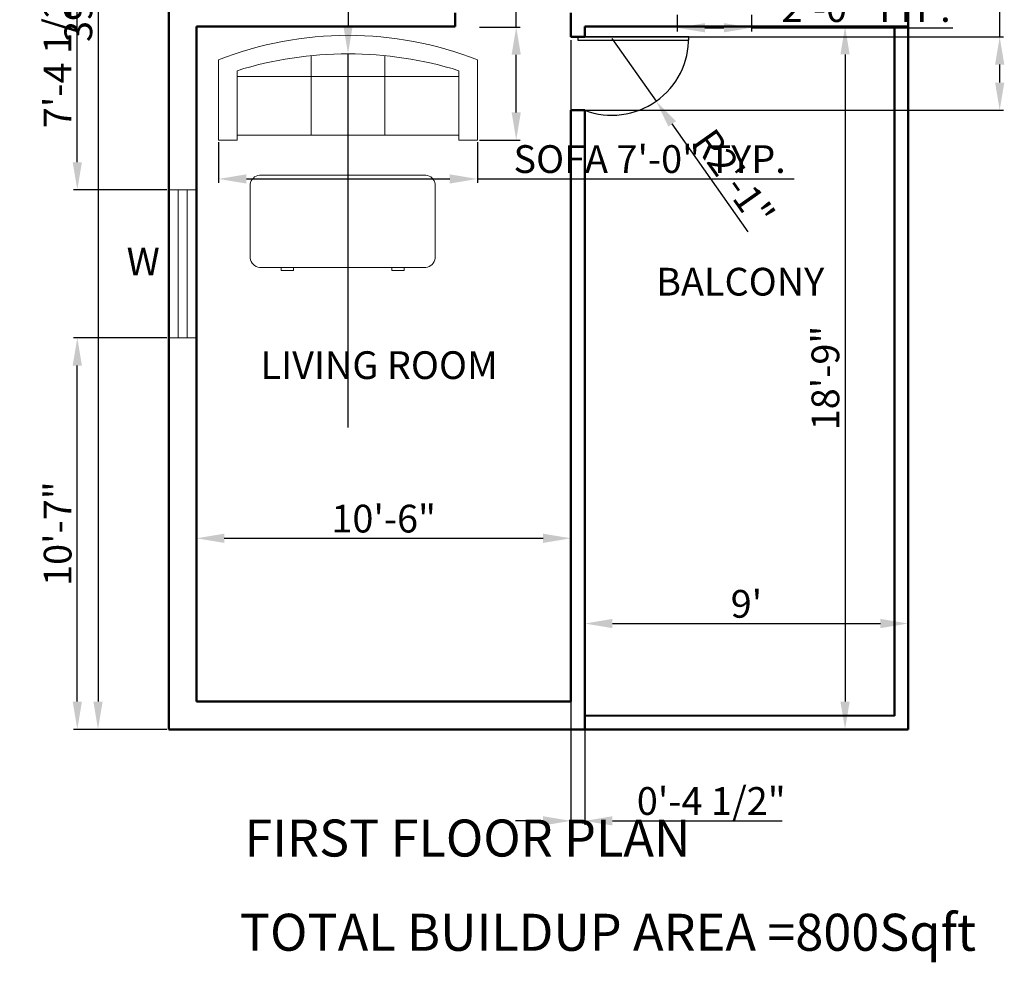
# Model space of a CAD drawing. Units: inches. Extents: x 1802 to 2621, y 1038 to 1686.
# Tile 4 of 5: x 2212 to 2532, y 1038 to 1344. Entities that reach past the tile are written whole.
import ezdxf

# ---------------------------------------------------------------- set-up
doc = ezdxf.new("R2010")
doc.units = ezdxf.units.IN
for name, color, linetype, lineweight in [('A-ANNO-DIMS', 2, 'Continuous', 18), ('A-ANNO-TEXT', 7, 'Continuous', 18), ('A-AREA-IDEN', 7, 'Continuous', 25), ('A-DOOR', 3, 'Continuous', 25), ('A-FURN', 8, 'Continuous', 18), ('A-GLAZ', 4, 'Continuous', 18), ('A-WALL', 7, 'Continuous', 50)]:
    doc.layers.add(name, color=color, linetype=linetype, lineweight=lineweight)
doc.styles.get("Standard").update_dxf_attribs({"font": 'arial.ttf'})
doc.dimstyles.new('ISO-25', dxfattribs={"dimtxt": 9, "dimasz": 9, "dimexe": 1.25, "dimexo": 0.625, "dimtad": 1, "dimdec": 1, "dimrnd": 9, "dimlunit": 3, "dimtxsty": 'Standard', "dimcen": 2.5, "dimadec": 0, "dimazin": 0, "dimtfac": 1, "dimtdec": 1, "dimtmove": 0, "dimatfit": 3, "dimfxl": 1, "dimarcsym": 0})

# ---------------------------------------------------------------- blocks, each defined once
blk = doc.blocks.new('*D22')
at = {"layer": 'A-ANNO-DIMS', "color": 0, "lineweight": -2, "transparency": 16777216}
for p, q in [((2259.93, 1593.56), (2236.33, 1593.56)), ((2237.58, 1584.56), (2237.58, 1122.56)), ((2259.93, 1113.56), (2236.33, 1113.56))]:
    blk.add_line(p, q, dxfattribs=at)
at = {"layer": 'A-ANNO-DIMS', "color": 0, "transparency": 16777216}
for points in [[(2236.08, 1584.56), (2239.08, 1584.56), (2237.58, 1593.56)], [(2236.08, 1122.56), (2239.08, 1122.56), (2237.58, 1113.56)]]:
    blk.add_solid(points, dxfattribs=at)
at = {"layer": 'Defpoints', "color": 0, "transparency": 16777216}
for p in [(2260.56, 1593.56), (2237.58, 1113.56), (2260.56, 1113.56)]:
    blk.add_point(p, dxfattribs=at)
at = {"layer": 'A-ANNO-DIMS', "color": 0, "transparency": 16777216, "insert": (2232.36, 1353.56), "char_height": 9, "attachment_point": 5, "rotation": 90}
blk.add_mtext('39\'-9"', dxfattribs=at)
blk = doc.blocks.new('*D25')
at = {"layer": 'A-ANNO-DIMS', "color": 0, "lineweight": -2, "transparency": 16777216}
for p, q in [((2269.56, 1123.18), (2269.56, 1176.79)), ((2391.06, 1123.18), (2391.06, 1176.79)), ((2278.56, 1175.54), (2382.06, 1175.54))]:
    blk.add_line(p, q, dxfattribs=at)
at = {"layer": 'A-ANNO-DIMS', "color": 0, "transparency": 16777216}
for points in [[(2278.56, 1177.04), (2278.56, 1174.04), (2269.56, 1175.54)], [(2382.06, 1177.04), (2382.06, 1174.04), (2391.06, 1175.54)]]:
    blk.add_solid(points, dxfattribs=at)
at = {"layer": 'Defpoints', "color": 0, "transparency": 16777216}
for p in [(2391.06, 1175.54), (2269.56, 1122.56), (2391.06, 1122.56)]:
    blk.add_point(p, dxfattribs=at)
at = {"layer": 'A-ANNO-DIMS', "color": 0, "transparency": 16777216, "insert": (2330.31, 1180.76), "char_height": 9, "attachment_point": 5}
blk.add_mtext('10\'-6"', dxfattribs=at)
blk = doc.blocks.new('Sofa - Roundback 7 ft.')
for p, q in [((-12.00002, -32.4421), (-12.00003, -6.5971)), ((11.99997, -32.4421), (11.99998, -6.5971)), ((-36.000027, -34), (-36.000027, -11.4696)), ((35.99998, -34), (35.99998, -11.4696)), ((-35.999844, -13.3819), (35.9998, -13.3819)), ((-36.000027, -32.4421), (35.99998, -32.4421))]:
    blk.add_line(p, q)
for points in [[(-36.000027, -34), (-42.000027, -34), (-42.000027, -8)], [(41.99998, -8), (41.99998, -34), (35.99998, -34)]]:
    blk.add_lwpolyline(points)
for centre, radius, start, end in [((0, -114.25), 114.25, 68.43141, 111.5686), ((-0.00001, -127.1968), 121.1968, 72.72033, 107.2797)]:
    blk.add_arc(centre, radius, start, end)
blk = doc.blocks.new('Desk - 30 x 60 in.')
for p, q in [((-26.999995, 0), (26.999995, 0)), ((-29.999995, -27), (-29.999995, -3)), ((29.999995, -3), (29.999995, -27)), ((26.999995, -30), (-26.999995, -30)), ((-20.000005, -30), (-20.000005, -31)), ((-20.000005, -31), (-16.000005, -31)), ((-16.000005, -31), (-16.000005, -30)), ((15.999995, -31), (15.999995, -30)), ((19.999995, -31), (15.999995, -31)), ((19.999995, -30), (19.999995, -31))]:
    blk.add_line(p, q)
for centre, start, end in [((-26.499995, -3.5), 98.1301, 171.8699), ((26.499995, -3.5), 8.130102, 81.8699), ((-26.499995, -26.5), 188.1301, 261.8699), ((26.499995, -26.5), 278.1301, 351.8699)]:
    blk.add_arc(centre, 3.535534, start, end)
blk = doc.blocks.new('*D27')
at = {"layer": 'A-ANNO-DIMS', "color": 0, "lineweight": -2, "transparency": 16777216}
for p, q in [((2395.56, 1114.18), (2395.56, 1149.14)), ((2404.56, 1147.89), (2491.56, 1147.89)), ((2500.56, 1114.18), (2500.56, 1149.14))]:
    blk.add_line(p, q, dxfattribs=at)
at = {"layer": 'A-ANNO-DIMS', "color": 0, "transparency": 16777216}
for points in [[(2404.56, 1149.39), (2404.56, 1146.39), (2395.56, 1147.89)], [(2491.56, 1149.39), (2491.56, 1146.39), (2500.56, 1147.89)]]:
    blk.add_solid(points, dxfattribs=at)
at = {"layer": 'Defpoints', "color": 0, "transparency": 16777216}
for p in [(2500.56, 1147.89), (2395.56, 1113.56), (2500.56, 1113.56)]:
    blk.add_point(p, dxfattribs=at)
at = {"layer": 'A-ANNO-DIMS', "color": 0, "transparency": 16777216, "insert": (2448.06, 1153.11), "char_height": 9, "attachment_point": 5}
blk.add_mtext("9'", dxfattribs=at)
blk = doc.blocks.new('*D28')
at = {"layer": 'A-ANNO-DIMS', "color": 0, "lineweight": -2, "transparency": 16777216}
for p, q in [((2499.93, 1341.56), (2478.81, 1341.56)), ((2480.06, 1332.56), (2480.06, 1122.56)), ((2499.93, 1113.56), (2478.81, 1113.56))]:
    blk.add_line(p, q, dxfattribs=at)
at = {"layer": 'A-ANNO-DIMS', "color": 0, "transparency": 16777216}
for points in [[(2478.56, 1332.56), (2481.56, 1332.56), (2480.06, 1341.56)], [(2478.56, 1122.56), (2481.56, 1122.56), (2480.06, 1113.56)]]:
    blk.add_solid(points, dxfattribs=at)
at = {"layer": 'Defpoints', "color": 0, "transparency": 16777216}
for p in [(2500.56, 1341.56), (2480.06, 1113.56), (2500.56, 1113.56)]:
    blk.add_point(p, dxfattribs=at)
at = {"layer": 'A-ANNO-DIMS', "color": 0, "transparency": 16777216, "insert": (2474.84, 1227.56), "char_height": 9, "attachment_point": 5, "rotation": 90}
blk.add_mtext('18\'-9"', dxfattribs=at)
blk = doc.blocks.new('WIN-48IN')
for p, q in [((9, 48), (0, 48)), ((3, 48), (3, 0)), ((6, 48), (6, 0)), ((9, 0), (0, 0))]:
    blk.add_line(p, q)
blk = doc.blocks.new('*D45')
at = {"layer": 'A-ANNO-DIMS', "color": 0, "lineweight": -2, "transparency": 16777216}
for p, q in [((2276.73, 1304.11), (2276.73, 1290.89)), ((2360.73, 1304.11), (2360.73, 1290.89)), ((2285.73, 1292.14), (2351.73, 1292.14)), ((2360.73, 1292.14), (2463.52, 1292.14))]:
    blk.add_line(p, q, dxfattribs=at)
at = {"layer": 'A-ANNO-DIMS', "color": 0, "transparency": 16777216}
for points in [[(2285.73, 1293.64), (2285.73, 1290.64), (2276.73, 1292.14)], [(2351.73, 1293.64), (2351.73, 1290.64), (2360.73, 1292.14)]]:
    blk.add_solid(points, dxfattribs=at)
at = {"layer": 'Defpoints', "color": 0, "transparency": 16777216}
for p in [(2276.73, 1304.74), (2360.73, 1304.74), (2360.73, 1292.14)]:
    blk.add_point(p, dxfattribs=at)
at = {"layer": 'A-ANNO-DIMS', "color": 0, "transparency": 16777216, "insert": (2416.63, 1297.42), "char_height": 9, "attachment_point": 5}
blk.add_mtext('SOFA 7\'-0" TYP.', dxfattribs=at)
blk = doc.blocks.new('*D46')
at = {"layer": 'A-ANNO-DIMS', "color": 0, "lineweight": -2, "transparency": 16777216}
for p, q in [((2373.33, 1341.41), (2373.33, 1427.48)), ((2361.36, 1341.41), (2374.58, 1341.41)), ((2373.33, 1313.74), (2373.33, 1332.41)), ((2361.36, 1304.74), (2374.58, 1304.74))]:
    blk.add_line(p, q, dxfattribs=at)
at = {"layer": 'A-ANNO-DIMS', "color": 0, "transparency": 16777216}
for points in [[(2371.83, 1332.41), (2374.83, 1332.41), (2373.33, 1341.41)], [(2371.83, 1313.74), (2374.83, 1313.74), (2373.33, 1304.74)]]:
    blk.add_solid(points, dxfattribs=at)
at = {"layer": 'Defpoints', "color": 0, "transparency": 16777216}
for p in [(2360.73, 1341.41), (2373.33, 1341.41), (2360.73, 1304.74)]:
    blk.add_point(p, dxfattribs=at)
at = {"layer": 'A-ANNO-DIMS', "color": 0, "transparency": 16777216, "insert": (2368.05, 1388.94), "char_height": 9, "attachment_point": 5, "rotation": 90}
blk.add_mtext('3\'-0 1/2" TYP.', dxfattribs=at)
blk = doc.blocks.new('*D54')
at = {"layer": 'A-ANNO-DIMS', "color": 0, "lineweight": -2, "transparency": 16777216}
for p, q in [((2425.56, 1345.43), (2425.56, 1339.95)), ((2449.75, 1345.43), (2449.75, 1339.95)), ((2434.56, 1341.2), (2440.75, 1341.2)), ((2449.75, 1341.2), (2515.01, 1341.2))]:
    blk.add_line(p, q, dxfattribs=at)
at = {"layer": 'A-ANNO-DIMS', "color": 0, "transparency": 16777216}
for points in [[(2434.56, 1342.7), (2434.56, 1339.7), (2425.56, 1341.2)], [(2440.75, 1342.7), (2440.75, 1339.7), (2449.75, 1341.2)]]:
    blk.add_solid(points, dxfattribs=at)
at = {"layer": 'Defpoints', "color": 0, "transparency": 16777216}
for p in [(2425.56, 1346.06), (2449.75, 1346.06), (2449.75, 1341.2)]:
    blk.add_point(p, dxfattribs=at)
at = {"layer": 'A-ANNO-DIMS', "color": 0, "transparency": 16777216, "insert": (2486.88, 1346.42), "char_height": 9, "attachment_point": 5}
blk.add_mtext('2\'-0" TYP.', dxfattribs=at)
blk = doc.blocks.new('*D66')
at = {"layer": 'A-ANNO-DIMS', "color": 0, "lineweight": -2, "transparency": 16777216}
for p, q in [((2391.06, 1313.78), (2391.06, 1082.61)), ((2395.56, 1313.78), (2395.56, 1082.61)), ((2382.06, 1083.86), (2373.06, 1083.86)), ((2391.06, 1083.86), (2395.56, 1083.86)), ((2404.56, 1083.86), (2459.7, 1083.86))]:
    blk.add_line(p, q, dxfattribs=at)
at = {"layer": 'A-ANNO-DIMS', "color": 0, "transparency": 16777216}
for points in [[(2382.06, 1085.36), (2382.06, 1082.36), (2391.06, 1083.86)], [(2404.56, 1085.36), (2404.56, 1082.36), (2395.56, 1083.86)]]:
    blk.add_solid(points, dxfattribs=at)
at = {"layer": 'Defpoints', "color": 0, "transparency": 16777216}
for p in [(2391.06, 1314.41), (2395.56, 1314.41), (2395.56, 1083.86)]:
    blk.add_point(p, dxfattribs=at)
at = {"layer": 'A-ANNO-DIMS', "color": 0, "transparency": 16777216, "insert": (2436.63, 1089.14), "char_height": 9, "attachment_point": 5}
blk.add_mtext('0\'-4 1/2"', dxfattribs=at)
blk = doc.blocks.new('*D67')
at = {"layer": 'A-ANNO-DIMS', "color": 0, "lineweight": -2, "transparency": 16777216}
for p, q in [((2259.93, 1240.57), (2229.61, 1240.57)), ((2230.86, 1122.56), (2230.86, 1231.57)), ((2259.93, 1113.56), (2229.61, 1113.56))]:
    blk.add_line(p, q, dxfattribs=at)
at = {"layer": 'A-ANNO-DIMS', "color": 0, "transparency": 16777216}
for points in [[(2229.36, 1231.57), (2232.36, 1231.57), (2230.86, 1240.57)], [(2229.36, 1122.56), (2232.36, 1122.56), (2230.86, 1113.56)]]:
    blk.add_solid(points, dxfattribs=at)
at = {"layer": 'Defpoints', "color": 0, "transparency": 16777216}
for p in [(2230.86, 1240.57), (2260.56, 1240.57), (2260.56, 1113.56)]:
    blk.add_point(p, dxfattribs=at)
at = {"layer": 'A-ANNO-DIMS', "color": 0, "transparency": 16777216, "insert": (2225.64, 1177.06), "char_height": 9, "attachment_point": 5, "rotation": 90}
blk.add_mtext('10\'-7"', dxfattribs=at)
blk = doc.blocks.new('*D68')
at = {"layer": 'A-ANNO-DIMS', "color": 0, "lineweight": -2, "transparency": 16777216}
for p, q in [((2259.93, 1377), (2229.61, 1377)), ((2230.86, 1297.57), (2230.86, 1368)), ((2259.93, 1288.57), (2229.61, 1288.57))]:
    blk.add_line(p, q, dxfattribs=at)
at = {"layer": 'A-ANNO-DIMS', "color": 0, "transparency": 16777216}
for points in [[(2229.36, 1368), (2232.36, 1368), (2230.86, 1377)], [(2229.36, 1297.57), (2232.36, 1297.57), (2230.86, 1288.57)]]:
    blk.add_solid(points, dxfattribs=at)
at = {"layer": 'Defpoints', "color": 0, "transparency": 16777216}
for p in [(2230.86, 1377), (2260.56, 1377), (2260.56, 1288.57)]:
    blk.add_point(p, dxfattribs=at)
at = {"layer": 'A-ANNO-DIMS', "color": 0, "transparency": 16777216, "insert": (2225.58, 1332.78), "char_height": 9, "attachment_point": 5, "rotation": 90}
blk.add_mtext('7\'-4 1/2"', dxfattribs=at)
blk = doc.blocks.new('*D76')
at = {"layer": 'A-ANNO-DIMS', "color": 0, "lineweight": -2, "transparency": 16777216}
for p, q in [((2530.26, 1338.22), (2530.26, 1372.54)), ((2391.68, 1338.22), (2531.51, 1338.22)), ((2530.26, 1323.41), (2530.26, 1329.22)), ((2391.68, 1314.41), (2531.51, 1314.41))]:
    blk.add_line(p, q, dxfattribs=at)
at = {"layer": 'A-ANNO-DIMS', "color": 0, "transparency": 16777216}
for points in [[(2528.76, 1329.22), (2531.76, 1329.22), (2530.26, 1338.22)], [(2528.76, 1323.41), (2531.76, 1323.41), (2530.26, 1314.41)]]:
    blk.add_solid(points, dxfattribs=at)
at = {"layer": 'Defpoints', "color": 0, "transparency": 16777216}
for p in [(2391.06, 1338.22), (2530.26, 1338.22), (2391.06, 1314.41)]:
    blk.add_point(p, dxfattribs=at)
at = {"layer": 'A-ANNO-DIMS', "color": 0, "transparency": 16777216, "insert": (2525.04, 1359.88), "char_height": 9, "attachment_point": 5, "rotation": 90}
blk.add_mtext('2\'-0"', dxfattribs=at)
blk = doc.blocks.new('*D80')
at = {"layer": 'A-ANNO-DIMS', "color": 0, "lineweight": -2, "transparency": 16777216}
for p, q in [((2404.39, 1337.72), (2418.75, 1317.35)), ((2448.61, 1275.03), (2423.94, 1310))]:
    blk.add_line(p, q, dxfattribs=at)
at = {"layer": 'A-ANNO-DIMS', "color": 0, "transparency": 16777216}
blk.add_solid([(2425.17, 1310.86), (2422.72, 1309.13), (2418.75, 1317.35)], dxfattribs=at)
at = {"layer": 'Defpoints', "color": 0, "transparency": 16777216}
for p in [(2404.39, 1337.72), (2418.75, 1317.35)]:
    blk.add_point(p, dxfattribs=at)
at = {"layer": 'A-ANNO-DIMS', "color": 0, "transparency": 16777216, "insert": (2443.07, 1291.8), "char_height": 9, "attachment_point": 5, "rotation": 305.1993}
blk.add_mtext('R2\'-1"', dxfattribs=at)
blk = doc.blocks.new('*D84')
at = {"layer": 'A-ANNO-DIMS', "color": 0, "lineweight": -2, "transparency": 16777216}
for p, q in [((2318.73, 1435.59), (2318.73, 1341.74)), ((2318.73, 1211.54), (2318.73, 1332.74))]:
    blk.add_line(p, q, dxfattribs=at)
at = {"layer": 'A-ANNO-DIMS', "color": 0, "transparency": 16777216}
blk.add_solid([(2320.23, 1341.74), (2317.23, 1341.74), (2318.73, 1332.74)], dxfattribs=at)
at = {"layer": 'Defpoints', "color": 0, "transparency": 16777216}
for p in [(2318.73, 1332.74), (2318.73, 1211.54)]:
    blk.add_point(p, dxfattribs=at)
at = {"layer": 'A-ANNO-DIMS', "color": 0, "transparency": 16777216, "insert": (2323.95, 1405.46), "char_height": 9, "attachment_point": 5, "rotation": 270.0001}
blk.add_mtext('2X R10\'-1"', dxfattribs=at)

msp = doc.modelspace()

# ---------------------------------------------------------------- linework, layer by layer
at = {"layer": 'A-DOOR'}
for p, q in [((2391.06, 1337.22), (2391.06, 1314.41)), ((2393.31, 1338.22), (2393.31, 1337.22)), ((2393.31, 1337.22), (2429.31, 1337.22)), ((2429.31, 1338.22), (2395.56, 1338.22)), ((2429.31, 1337.22), (2429.31, 1338.22))]:
    msp.add_line(p, q, dxfattribs=at)
msp.add_arc((2404.39, 1337.72), 24.92, 249.25, 1.1495, dxfattribs=at)
at = {"layer": 'A-WALL'}
for p, q in [((2260.56, 1593.56), (2260.56, 1113.56)), ((2500.56, 1113.56), (2500.56, 1593.56)), ((2353.56, 1346.06), (2353.56, 1341.56)), ((2391.06, 1341.56), (2391.06, 1346.06)), ((2269.56, 1341.56), (2269.56, 1122.56)), ((2353.56, 1341.56), (2269.56, 1341.56)), ((2391.06, 1338.22), (2391.06, 1341.56)), ((2425.56, 1341.56), (2395.56, 1341.56)), ((2395.56, 1338.22), (2395.56, 1341.56)), ((2425.56, 1341.56), (2430.06, 1341.56)), ((2491.56, 1341.56), (2430.06, 1341.56)), ((2491.56, 1341.56), (2500.56, 1341.56)), ((2496.06, 1341.56), (2496.06, 1117.94)), ((2391.06, 1338.22), (2395.56, 1338.22)), ((2391.06, 1122.56), (2391.06, 1314.41)), ((2395.56, 1314.41), (2391.06, 1314.41)), ((2395.56, 1122.56), (2395.56, 1314.41)), ((2269.56, 1122.56), (2277.66, 1122.56)), ((2277.66, 1122.56), (2325.66, 1122.56)), ((2325.66, 1122.56), (2391.06, 1122.56)), ((2395.56, 1122.56), (2395.56, 1113.56)), ((2496.06, 1117.94), (2395.56, 1118.06)), ((2260.56, 1113.56), (2277.66, 1113.56)), ((2277.66, 1113.56), (2325.66, 1113.56)), ((2325.66, 1113.56), (2500.56, 1113.56))]:
    msp.add_line(p, q, dxfattribs=at)

# ---------------------------------------------------------------- block references
at = {"layer": 'A-FURN'}
for name, p in [('Sofa - Roundback 7 ft.', (2318.73, 1338.74)), ('Desk - 30 x 60 in.', (2317, 1293.41))]:
    msp.add_blockref(name, p, dxfattribs=at)
at = {"layer": 'A-GLAZ', "rotation": 180}
msp.add_blockref('WIN-48IN', (2269.56, 1288.57), dxfattribs=at)

# ---------------------------------------------------------------- texts
at = {"layer": 'A-ANNO-TEXT', "attachment_point": 1}
for s, width, insert, char_height in [('W', 30.0361, (2246.86, 1269.86), 9), ('FIRST FLOOR PLAN', 217.7869, (2285.1, 1084.29), 12)]:
    msp.add_mtext_dynamic_manual_height_columns(s, width=width, gutter_width=12.5, heights=[0], dxfattribs=dict(at, insert=insert, char_height=char_height))
at = {"layer": 'A-AREA-IDEN', "attachment_point": 1}
for s, width, insert, char_height in [('BALCONY', 82.6611, (2418.75, 1263.3), 9), ('LIVING ROOM', 82.6611, (2290.33, 1236.22), 9), ('TOTAL BUILDUP AREA =800Sqft', 278.6904, (2283.61, 1053.72), 12)]:
    msp.add_mtext_dynamic_manual_height_columns(s, width=width, gutter_width=12.5, heights=[0], dxfattribs=dict(at, insert=insert, char_height=char_height))

# ---------------------------------------------------------------- dimensions: what is measured, and where the dimension line sits
at = {"layer": 'A-ANNO-DIMS'}
for base, p1, p2, override, picture, middle in [((2237.58, 1113.56), (2260.56, 1593.56), (2260.56, 1113.56), {"dimclrd": 0, "dimclre": 0, "dimclrt": 0}, '*D22', (2232.36, 1353.56)), ((2230.86, 1377), (2260.56, 1288.57), (2260.56, 1377), {"dimdec": 1, "dimlfac": 1, "dimrnd": 0, "dimzin": 1, "dimdsep": 46, "dimlunit": 4, "dimfrac": 2}, '*D68', (2225.58, 1332.78)), ((2530.26, 1338.22), (2391.06, 1314.41), (2391.06, 1338.22), {"dimdec": 1, "dimlfac": 1, "dimrnd": 0, "dimzin": 1, "dimdsep": 46, "dimlunit": 4, "dimfrac": 2}, '*D76', (2525.04, 1359.88)), ((2480.06, 1113.56), (2500.56, 1341.56), (2500.56, 1113.56), {"dimclrd": 0, "dimclre": 0, "dimclrt": 0}, '*D28', (2474.84, 1227.56)), ((2230.86, 1240.57), (2260.56, 1113.56), (2260.56, 1240.57), {"dimdec": 1, "dimlfac": 1, "dimrnd": 0, "dimzin": 1, "dimdsep": 46, "dimlunit": 4, "dimfrac": 2}, '*D67', (2225.64, 1177.06))]:
    dim = msp.add_linear_dim(base=base, p1=p1, p2=p2, angle=90, dimstyle='ISO-25', override=override, dxfattribs=at)
    dim.commit()
    dim.dimension.update_dxf_attribs({"geometry": picture, "text_midpoint": middle})
dim = msp.add_radius_dim(center=(2318.73, 1211.54), mpoint=(2318.73, 1332.74), text='2X <>', dimstyle='ISO-25', override={"dimdec": 1, "dimlfac": 1, "dimrnd": 0, "dimzin": 1, "dimdsep": 46, "dimlunit": 4, "dimfrac": 2}, dxfattribs=at)
dim.commit()
dim.dimension.update_dxf_attribs({"geometry": '*D84', "text_midpoint": (2318.73, 1405.46), "dimtype": 164})
dim = msp.add_linear_dim(base=(2373.33, 1341.41), p1=(2360.73, 1304.74), p2=(2360.73, 1341.41), angle=90, text='<> TYP.', dimstyle='ISO-25', override={"dimdec": 1, "dimlfac": 1, "dimrnd": 0, "dimzin": 1, "dimdsep": 46, "dimlunit": 4, "dimfrac": 2}, dxfattribs=at)
dim.commit()
dim.dimension.update_dxf_attribs({"geometry": '*D46', "text_midpoint": (2368.05, 1388.94)})
for base, p1, p2, text, picture, middle in [((2449.75, 1341.2), (2425.56, 1346.06), (2449.75, 1346.06), '<> TYP.', '*D54', (2486.88, 1346.42)), ((2360.73, 1292.14), (2276.73, 1304.74), (2360.73, 1304.74), 'SOFA <> TYP.', '*D45', (2416.63, 1297.42))]:
    dim = msp.add_linear_dim(base=base, p1=p1, p2=p2, text=text, dimstyle='ISO-25', override={"dimdec": 1, "dimlfac": 1, "dimrnd": 0, "dimzin": 1, "dimdsep": 46, "dimlunit": 4, "dimfrac": 2}, dxfattribs=at)
    dim.commit()
    dim.dimension.update_dxf_attribs({"geometry": picture, "text_midpoint": middle})
dim = msp.add_radius_dim(center=(2404.39, 1337.72), mpoint=(2418.75, 1317.35), dimstyle='ISO-25', override={"dimdec": 1, "dimlfac": 1, "dimrnd": 0, "dimzin": 1, "dimdsep": 46, "dimlunit": 4, "dimfrac": 2}, dxfattribs=at)
dim.commit()
dim.dimension.update_dxf_attribs({"geometry": '*D80', "text_midpoint": (2443.07, 1291.8)})
for base, p1, p2, override, picture, middle in [((2395.56, 1083.86), (2391.06, 1314.41), (2395.56, 1314.41), {"dimdec": 1, "dimlfac": 1, "dimrnd": 0, "dimzin": 1, "dimdsep": 46, "dimlunit": 4, "dimfrac": 2}, '*D66', (2436.63, 1089.14)), ((2391.06, 1175.54), (2269.56, 1122.56), (2391.06, 1122.56), {"dimclrd": 0, "dimclre": 0, "dimclrt": 0}, '*D25', (2330.31, 1180.76)), ((2500.56, 1147.89), (2395.56, 1113.56), (2500.56, 1113.56), {"dimclrd": 0, "dimclre": 0, "dimclrt": 0}, '*D27', (2448.06, 1153.11))]:
    dim = msp.add_linear_dim(base=base, p1=p1, p2=p2, dimstyle='ISO-25', override=override, dxfattribs=at)
    dim.commit()
    dim.dimension.update_dxf_attribs({"geometry": picture, "text_midpoint": middle})

doc.saveas('drawing.dxf')
